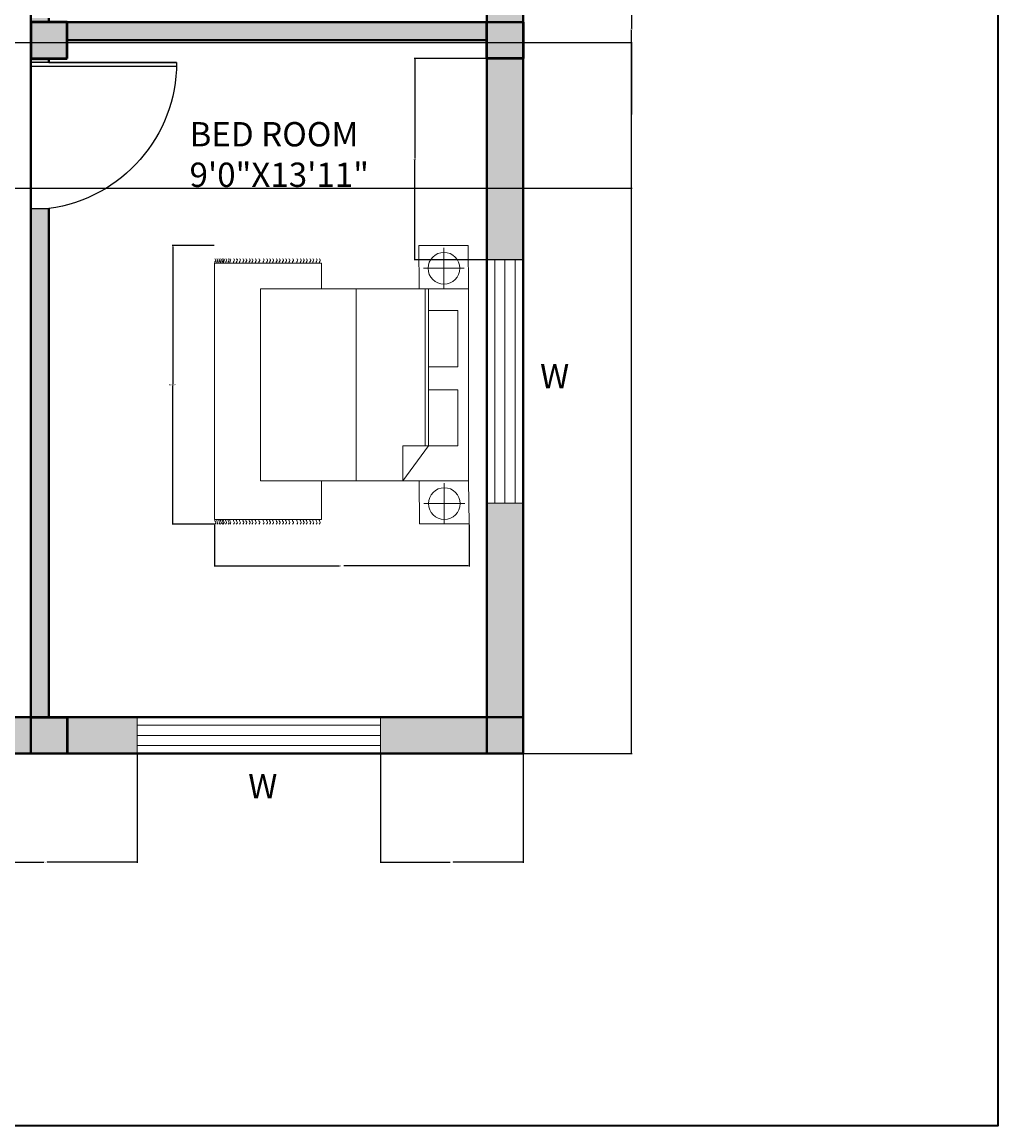
# Model space of a CAD drawing. Units: inches. Extents: x 25176543 to 25177243, y 80295576 to 80296086.
# Tile 6 of 11: x 25177002 to 25177243, y 80295576 to 80295848. Entities that reach past the tile are written whole.
import ezdxf

# ---------------------------------------------------------------- set-up
doc = ezdxf.new("R2010")
doc.units = ezdxf.units.IN
doc.header["$MEASUREMENT"] = 0
for name, color, linetype, lineweight in [('A-ANNO-DIMS', 2, 'Continuous', 18), ('A-ANNO-IDEN', 7, 'Continuous', 18), ('A-ANNO-TTLB', 7, 'Continuous', 35), ('A-AREA-IDEN', 7, 'Continuous', 18), ('A-COLS', 7, 'Continuous', 50), ('A-COLS-PATT', 251, 'Continuous', 13), ('A-DOOR', 3, 'Continuous', 25), ('A-GLAZ', 4, 'Continuous', 18), ('A-WALL', 7, 'Continuous', 40), ('A-WALL-PATT', 146, 'Continuous', 13), ('furniture', 31, 'Continuous', 13)]:
    doc.layers.add(name, color=color, linetype=linetype, lineweight=lineweight)
doc.styles.get("Standard").update_dxf_attribs({"font": 'arial.ttf'})
doc.dimstyles.get("Standard").update_dxf_attribs({"dimtxt": 0.18, "dimasz": 0.18, "dimexe": 0.18, "dimexo": 0.0625, "dimgap": 0.09, "dimtad": 0, "dimtih": 1, "dimtoh": 1, "dimdec": 4, "dimzin": 0, "dimdsep": 46, "dimtxsty": 'Standard', "dimcen": 0.09, "dimadec": 0, "dimazin": 0, "dimtfac": 1, "dimtdec": 4, "dimtofl": 0, "dimtmove": 0, "dimatfit": 3, "dimfxl": 1, "dimtolj": 1, "dimtzin": 0, "dimarcsym": 0})

# ---------------------------------------------------------------- blocks, each defined once
blk = doc.blocks.new('BED-DOUBLE-WITH-NIGHTSTANDS')
for p, q in [((5.6, 61.62), (5.6, 51.56)), ((63.65, 61.72), (63.65, 51.66)), ((10.63, 56.59), (0.57, 56.59)), ((68.68, 56.69), (58.62, 56.69)), ((49.39, 52.82), (10.63, 52.82)), ((49.44, 52), (10.63, 52)), ((49.39, 52.82), (58, 46.47)), ((49.44, 52.82), (49.44, 46.47)), ((49.44, 46.47), (58, 46.47)), ((58.05, 34.96), (10.63, 34.96)), ((4.35, 0), (4.35, 26.37)), ((4.35, 26.37), (10.65, 26.37)), ((58.05, 26.37), (67.59, 26.37)), ((67.59, 26.37), (67.59, 0)), ((67.59, 0), (4.35, 0))]:
    blk.add_line(p, q)
for points in [[(0, 50.39), (10.63, 50.5), (10.63, 62.68), (0, 62.58)], [(58.05, 62.68), (58.05, 11.37), (10.63, 11.37), (10.63, 62.68)], [(58.05, 50.5), (68.68, 50.6), (68.68, 62.78), (58.05, 62.68)], [(29.88, 59.98), (29.88, 52.82), (15.98, 52.82), (15.98, 59.98)], [(49.44, 59.98), (49.44, 52.82), (35.55, 52.82), (35.55, 59.98)]]:
    blk.add_lwpolyline(points, close=True)
for centre in [(5.6, 56.59), (63.65, 56.69)]:
    blk.add_circle(centre, 3.92)
for points, knots in [([(3.23, 25.84), (3.32, 25.96), (3.52, 26.2), (3.86, 25.96), (4.14, 25.78), (4.29, 25.89), (4.35, 25.94)], [0, 0, 0, 0, 0.400747, 0.791423, 1.067667, 1.29709, 1.29709, 1.29709, 1.29709]), ([(3.23, 25.06), (3.32, 25.18), (3.52, 25.42), (3.86, 25.18), (4.14, 25.01), (4.29, 25.11), (4.35, 25.16)], [0, 0, 0, 0, 0.400747, 0.791423, 1.067667, 1.29709, 1.29709, 1.29709, 1.29709]), ([(3.23, 24.24), (3.32, 24.36), (3.52, 24.6), (3.86, 24.36), (4.14, 24.19), (4.29, 24.3), (4.35, 24.34)], [0, 0, 0, 0, 0.400747, 0.791423, 1.067667, 1.29709, 1.29709, 1.29709, 1.29709]), ([(68.71, 25.84), (68.61, 25.96), (68.42, 26.2), (68.08, 25.96), (67.8, 25.78), (67.65, 25.89), (67.58, 25.94)], [0, 0, 0, 0, 0.400747, 0.791423, 1.067667, 1.29709, 1.29709, 1.29709, 1.29709]), ([(68.71, 25.06), (68.61, 25.18), (68.42, 25.42), (68.08, 25.18), (67.8, 25.01), (67.65, 25.11), (67.58, 25.16)], [0, 0, 0, 0, 0.400747, 0.791423, 1.067667, 1.29709, 1.29709, 1.29709, 1.29709]), ([(68.71, 24.24), (68.61, 24.36), (68.42, 24.6), (68.08, 24.36), (67.8, 24.19), (67.65, 24.3), (67.58, 24.34)], [0, 0, 0, 0, 0.400747, 0.791423, 1.067667, 1.29709, 1.29709, 1.29709, 1.29709]), ([(3.23, 23.51), (3.32, 23.63), (3.52, 23.87), (3.86, 23.63), (4.14, 23.46), (4.29, 23.57), (4.35, 23.62)], [0, 0, 0, 0, 0.400747, 0.791423, 1.067667, 1.29709, 1.29709, 1.29709, 1.29709]), ([(3.23, 22.63), (3.32, 22.75), (3.52, 22.99), (3.86, 22.75), (4.14, 22.58), (4.29, 22.69), (4.35, 22.73)], [0, 0, 0, 0, 0.400747, 0.791423, 1.067667, 1.29709, 1.29709, 1.29709, 1.29709]), ([(3.23, 21.88), (3.32, 22), (3.52, 22.24), (3.86, 22), (4.14, 21.83), (4.29, 21.93), (4.35, 21.98)], [0, 0, 0, 0, 0.400747, 0.791423, 1.067667, 1.29709, 1.29709, 1.29709, 1.29709]), ([(68.71, 23.51), (68.61, 23.63), (68.42, 23.87), (68.08, 23.63), (67.8, 23.46), (67.65, 23.57), (67.58, 23.62)], [0, 0, 0, 0, 0.400747, 0.791423, 1.067667, 1.29709, 1.29709, 1.29709, 1.29709]), ([(68.71, 22.63), (68.61, 22.75), (68.42, 22.99), (68.08, 22.75), (67.8, 22.58), (67.65, 22.69), (67.58, 22.73)], [0, 0, 0, 0, 0.400747, 0.791423, 1.067667, 1.29709, 1.29709, 1.29709, 1.29709]), ([(68.71, 21.88), (68.61, 22), (68.42, 22.24), (68.08, 22), (67.8, 21.83), (67.65, 21.93), (67.58, 21.98)], [0, 0, 0, 0, 0.400747, 0.791423, 1.067667, 1.29709, 1.29709, 1.29709, 1.29709]), ([(3.23, 21.15), (3.32, 21.27), (3.52, 21.51), (3.86, 21.27), (4.14, 21.1), (4.29, 21.21), (4.35, 21.25)], [0, 0, 0, 0, 0.400747, 0.791423, 1.067667, 1.29709, 1.29709, 1.29709, 1.29709]), ([(3.23, 20.27), (3.32, 20.39), (3.52, 20.63), (3.86, 20.39), (4.14, 20.22), (4.29, 20.32), (4.35, 20.37)], [0, 0, 0, 0, 0.400747, 0.791423, 1.067667, 1.29709, 1.29709, 1.29709, 1.29709]), ([(3.23, 19.23), (3.32, 19.35), (3.52, 19.59), (3.86, 19.35), (4.14, 19.18), (4.29, 19.29), (4.35, 19.33)], [0, 0, 0, 0, 0.400747, 0.791423, 1.067667, 1.29709, 1.29709, 1.29709, 1.29709]), ([(68.71, 21.15), (68.61, 21.27), (68.42, 21.51), (68.08, 21.27), (67.8, 21.1), (67.65, 21.21), (67.58, 21.25)], [0, 0, 0, 0, 0.400747, 0.791423, 1.067667, 1.29709, 1.29709, 1.29709, 1.29709]), ([(68.71, 20.27), (68.61, 20.39), (68.42, 20.63), (68.08, 20.39), (67.8, 20.22), (67.65, 20.32), (67.58, 20.37)], [0, 0, 0, 0, 0.400747, 0.791423, 1.067667, 1.29709, 1.29709, 1.29709, 1.29709]), ([(68.71, 19.23), (68.61, 19.35), (68.42, 19.59), (68.08, 19.35), (67.8, 19.18), (67.65, 19.29), (67.58, 19.33)], [0, 0, 0, 0, 0.400747, 0.791423, 1.067667, 1.29709, 1.29709, 1.29709, 1.29709]), ([(3.23, 18.35), (3.32, 18.47), (3.52, 18.71), (3.86, 18.47), (4.14, 18.3), (4.29, 18.4), (4.35, 18.45)], [0, 0, 0, 0, 0.400747, 0.791423, 1.067667, 1.29709, 1.29709, 1.29709, 1.29709]), ([(3.23, 17.53), (3.32, 17.65), (3.52, 17.89), (3.86, 17.65), (4.14, 17.48), (4.29, 17.59), (4.35, 17.64)], [0, 0, 0, 0, 0.400747, 0.791423, 1.067667, 1.29709, 1.29709, 1.29709, 1.29709]), ([(3.23, 16.76), (3.32, 16.88), (3.52, 17.12), (3.86, 16.88), (4.14, 16.7), (4.29, 16.81), (4.35, 16.86)], [0, 0, 0, 0, 0.400747, 0.791423, 1.067667, 1.29709, 1.29709, 1.29709, 1.29709]), ([(68.71, 18.35), (68.61, 18.47), (68.42, 18.71), (68.08, 18.47), (67.8, 18.3), (67.65, 18.4), (67.58, 18.45)], [0, 0, 0, 0, 0.400747, 0.791423, 1.067667, 1.29709, 1.29709, 1.29709, 1.29709]), ([(68.71, 17.53), (68.61, 17.65), (68.42, 17.89), (68.08, 17.65), (67.8, 17.48), (67.65, 17.59), (67.58, 17.64)], [0, 0, 0, 0, 0.400747, 0.791423, 1.067667, 1.29709, 1.29709, 1.29709, 1.29709]), ([(68.71, 16.76), (68.61, 16.88), (68.42, 17.12), (68.08, 16.88), (67.8, 16.7), (67.65, 16.81), (67.58, 16.86)], [0, 0, 0, 0, 0.400747, 0.791423, 1.067667, 1.29709, 1.29709, 1.29709, 1.29709]), ([(3.23, 15.94), (3.32, 16.06), (3.52, 16.3), (3.86, 16.06), (4.14, 15.89), (4.29, 16), (4.35, 16.04)], [0, 0, 0, 0, 0.400747, 0.791423, 1.067667, 1.29709, 1.29709, 1.29709, 1.29709]), ([(3.23, 15.21), (3.32, 15.33), (3.52, 15.57), (3.86, 15.33), (4.14, 15.16), (4.29, 15.27), (4.35, 15.32)], [0, 0, 0, 0, 0.400747, 0.791423, 1.067667, 1.29709, 1.29709, 1.29709, 1.29709]), ([(3.23, 14.33), (3.32, 14.45), (3.52, 14.69), (3.86, 14.45), (4.14, 14.28), (4.29, 14.38), (4.35, 14.43)], [0, 0, 0, 0, 0.400747, 0.791423, 1.067667, 1.29709, 1.29709, 1.29709, 1.29709]), ([(3.23, 13.58), (3.32, 13.7), (3.52, 13.94), (3.86, 13.7), (4.14, 13.53), (4.29, 13.63), (4.35, 13.68)], [0, 0, 0, 0, 0.400747, 0.791423, 1.067667, 1.29709, 1.29709, 1.29709, 1.29709]), ([(68.71, 15.94), (68.61, 16.06), (68.42, 16.3), (68.08, 16.06), (67.8, 15.89), (67.65, 16), (67.58, 16.04)], [0, 0, 0, 0, 0.400747, 0.791423, 1.067667, 1.29709, 1.29709, 1.29709, 1.29709]), ([(68.71, 15.21), (68.61, 15.33), (68.42, 15.57), (68.08, 15.33), (67.8, 15.16), (67.65, 15.27), (67.58, 15.32)], [0, 0, 0, 0, 0.400747, 0.791423, 1.067667, 1.29709, 1.29709, 1.29709, 1.29709]), ([(68.71, 14.33), (68.61, 14.45), (68.42, 14.69), (68.08, 14.45), (67.8, 14.28), (67.65, 14.38), (67.58, 14.43)], [0, 0, 0, 0, 0.400747, 0.791423, 1.067667, 1.29709, 1.29709, 1.29709, 1.29709]), ([(68.71, 13.58), (68.61, 13.7), (68.42, 13.94), (68.08, 13.7), (67.8, 13.53), (67.65, 13.63), (67.58, 13.68)], [0, 0, 0, 0, 0.400747, 0.791423, 1.067667, 1.29709, 1.29709, 1.29709, 1.29709]), ([(3.23, 12.85), (3.32, 12.97), (3.52, 13.21), (3.86, 12.97), (4.14, 12.8), (4.29, 12.9), (4.35, 12.95)], [0, 0, 0, 0, 0.400747, 0.791423, 1.067667, 1.29709, 1.29709, 1.29709, 1.29709]), ([(3.23, 11.97), (3.32, 12.09), (3.52, 12.33), (3.86, 12.09), (4.14, 11.92), (4.29, 12.02), (4.35, 12.07)], [0, 0, 0, 0, 0.400747, 0.791423, 1.067667, 1.29709, 1.29709, 1.29709, 1.29709]), ([(3.23, 10.93), (3.32, 11.05), (3.52, 11.29), (3.86, 11.05), (4.14, 10.88), (4.29, 10.99), (4.35, 11.03)], [0, 0, 0, 0, 0.400747, 0.791423, 1.067667, 1.29709, 1.29709, 1.29709, 1.29709]), ([(68.71, 12.85), (68.61, 12.97), (68.42, 13.21), (68.08, 12.97), (67.8, 12.8), (67.65, 12.9), (67.58, 12.95)], [0, 0, 0, 0, 0.400747, 0.791423, 1.067667, 1.29709, 1.29709, 1.29709, 1.29709]), ([(68.71, 11.97), (68.61, 12.09), (68.42, 12.33), (68.08, 12.09), (67.8, 11.92), (67.65, 12.02), (67.58, 12.07)], [0, 0, 0, 0, 0.400747, 0.791423, 1.067667, 1.29709, 1.29709, 1.29709, 1.29709]), ([(68.71, 10.93), (68.61, 11.05), (68.42, 11.29), (68.08, 11.05), (67.8, 10.88), (67.65, 10.99), (67.58, 11.03)], [0, 0, 0, 0, 0.400747, 0.791423, 1.067667, 1.29709, 1.29709, 1.29709, 1.29709]), ([(3.23, 10.05), (3.32, 10.17), (3.52, 10.41), (3.86, 10.17), (4.14, 10), (4.29, 10.1), (4.35, 10.15)], [0, 0, 0, 0, 0.400747, 0.791423, 1.067667, 1.29709, 1.29709, 1.29709, 1.29709]), ([(3.23, 9.23), (3.32, 9.35), (3.52, 9.59), (3.86, 9.35), (4.14, 9.18), (4.29, 9.29), (4.35, 9.34)], [0, 0, 0, 0, 0.400747, 0.791423, 1.067667, 1.29709, 1.29709, 1.29709, 1.29709]), ([(3.23, 8.54), (3.32, 8.66), (3.52, 8.9), (3.86, 8.66), (4.14, 8.49), (4.29, 8.6), (4.35, 8.65)], [0, 0, 0, 0, 0.400747, 0.791423, 1.067667, 1.29709, 1.29709, 1.29709, 1.29709]), ([(68.71, 10.05), (68.61, 10.17), (68.42, 10.41), (68.08, 10.17), (67.8, 10), (67.65, 10.1), (67.58, 10.15)], [0, 0, 0, 0, 0.400747, 0.791423, 1.067667, 1.29709, 1.29709, 1.29709, 1.29709]), ([(68.71, 9.23), (68.61, 9.35), (68.42, 9.59), (68.08, 9.35), (67.8, 9.18), (67.65, 9.29), (67.58, 9.34)], [0, 0, 0, 0, 0.400747, 0.791423, 1.067667, 1.29709, 1.29709, 1.29709, 1.29709]), ([(68.71, 8.54), (68.61, 8.66), (68.42, 8.9), (68.08, 8.66), (67.8, 8.49), (67.65, 8.6), (67.58, 8.65)], [0, 0, 0, 0, 0.400747, 0.791423, 1.067667, 1.29709, 1.29709, 1.29709, 1.29709]), ([(3.23, 7.73), (3.32, 7.85), (3.52, 8.09), (3.86, 7.85), (4.14, 7.68), (4.29, 7.78), (4.35, 7.83)], [0, 0, 0, 0, 0.400747, 0.791423, 1.067667, 1.29709, 1.29709, 1.29709, 1.29709]), ([(3.23, 7), (3.32, 7.12), (3.52, 7.36), (3.86, 7.12), (4.14, 6.95), (4.29, 7.05), (4.35, 7.1)], [0, 0, 0, 0, 0.400747, 0.791423, 1.067667, 1.29709, 1.29709, 1.29709, 1.29709]), ([(3.23, 6.12), (3.32, 6.24), (3.52, 6.48), (3.86, 6.24), (4.14, 6.07), (4.29, 6.17), (4.35, 6.22)], [0, 0, 0, 0, 0.400747, 0.791423, 1.067667, 1.29709, 1.29709, 1.29709, 1.29709]), ([(3.23, 5.36), (3.32, 5.49), (3.52, 5.73), (3.86, 5.49), (4.14, 5.31), (4.29, 5.42), (4.35, 5.47)], [0, 0, 0, 0, 0.400747, 0.791423, 1.067667, 1.29709, 1.29709, 1.29709, 1.29709]), ([(68.71, 7.73), (68.61, 7.85), (68.42, 8.09), (68.08, 7.85), (67.8, 7.68), (67.65, 7.78), (67.58, 7.83)], [0, 0, 0, 0, 0.400747, 0.791423, 1.067667, 1.29709, 1.29709, 1.29709, 1.29709]), ([(68.71, 7), (68.61, 7.12), (68.42, 7.36), (68.08, 7.12), (67.8, 6.95), (67.65, 7.05), (67.58, 7.1)], [0, 0, 0, 0, 0.400747, 0.791423, 1.067667, 1.29709, 1.29709, 1.29709, 1.29709]), ([(68.71, 6.12), (68.61, 6.24), (68.42, 6.48), (68.08, 6.24), (67.8, 6.07), (67.65, 6.17), (67.58, 6.22)], [0, 0, 0, 0, 0.400747, 0.791423, 1.067667, 1.29709, 1.29709, 1.29709, 1.29709]), ([(68.71, 5.36), (68.61, 5.49), (68.42, 5.73), (68.08, 5.49), (67.8, 5.31), (67.65, 5.42), (67.58, 5.47)], [0, 0, 0, 0, 0.400747, 0.791423, 1.067667, 1.29709, 1.29709, 1.29709, 1.29709]), ([(3.23, 4.64), (3.32, 4.76), (3.52, 5), (3.86, 4.76), (4.14, 4.59), (4.29, 4.69), (4.35, 4.74)], [0, 0, 0, 0, 0.400747, 0.791423, 1.067667, 1.29709, 1.29709, 1.29709, 1.29709]), ([(3.23, 3.75), (3.32, 3.88), (3.52, 4.12), (3.86, 3.88), (4.14, 3.7), (4.29, 3.81), (4.35, 3.86)], [0, 0, 0, 0, 0.400747, 0.791423, 1.067667, 1.29709, 1.29709, 1.29709, 1.29709]), ([(3.23, 3.33), (3.32, 3.45), (3.52, 3.7), (3.86, 3.44), (4.14, 3.27), (4.29, 3.38), (4.35, 3.43)], [0, 0, 0, 0, 0.407265, 0.802015, 1.07826, 1.307683, 1.307683, 1.307683, 1.307683]), ([(3.23, 2.76), (3.32, 2.88), (3.52, 3.12), (3.86, 2.88), (4.14, 2.71), (4.29, 2.81), (4.35, 2.86)], [0, 0, 0, 0, 0.400747, 0.791423, 1.067667, 1.29709, 1.29709, 1.29709, 1.29709]), ([(68.71, 4.64), (68.61, 4.76), (68.42, 5), (68.08, 4.76), (67.8, 4.59), (67.66, 4.69), (67.59, 4.73)], [0, 0, 0, 0, 0.400747, 0.791423, 1.067667, 1.283686, 1.283686, 1.283686, 1.283686]), ([(68.71, 3.75), (68.61, 3.88), (68.42, 4.11), (68.08, 3.88), (67.8, 3.7), (67.66, 3.81), (67.59, 3.85)], [0, 0, 0, 0, 0.400747, 0.791423, 1.067667, 1.283686, 1.283686, 1.283686, 1.283686]), ([(68.71, 3.33), (68.61, 3.45), (68.42, 3.69), (68.08, 3.45), (67.8, 3.27), (67.66, 3.38), (67.59, 3.42)], [0, 0, 0, 0, 0.402903, 0.794912, 1.071156, 1.287177, 1.287177, 1.287177, 1.287177]), ([(68.71, 2.73), (68.61, 2.85), (68.42, 3.09), (68.08, 2.85), (67.8, 2.68), (67.66, 2.78), (67.59, 2.82)], [0, 0, 0, 0, 0.400747, 0.791423, 1.067667, 1.283686, 1.283686, 1.283686, 1.283686]), ([(3.23, 2.18), (3.32, 2.31), (3.52, 2.55), (3.86, 2.31), (4.14, 2.13), (4.29, 2.24), (4.35, 2.29)], [0, 0, 0, 0, 0.400747, 0.791423, 1.067667, 1.29709, 1.29709, 1.29709, 1.29709]), ([(3.23, 1.88), (3.32, 2), (3.52, 2.24), (3.86, 2), (4.14, 1.82), (4.29, 1.93), (4.35, 1.98)], [0, 0, 0, 0, 0.400747, 0.791423, 1.067667, 1.29709, 1.29709, 1.29709, 1.29709]), ([(3.23, 1.46), (3.32, 1.58), (3.52, 1.82), (3.86, 1.58), (4.14, 1.41), (4.29, 1.51), (4.35, 1.56)], [0, 0, 0, 0, 0.400747, 0.791423, 1.067667, 1.29709, 1.29709, 1.29709, 1.29709]), ([(3.23, 1.06), (3.32, 1.18), (3.52, 1.42), (3.86, 1.18), (4.14, 1.01), (4.29, 1.11), (4.35, 1.16)], [0, 0, 0, 0, 0.400747, 0.791423, 1.067667, 1.29709, 1.29709, 1.29709, 1.29709]), ([(3.23, 0.57), (3.32, 0.7), (3.52, 0.94), (3.86, 0.7), (4.14, 0.52), (4.29, 0.63), (4.35, 0.68)], [0, 0, 0, 0, 0.400747, 0.791423, 1.067667, 1.29709, 1.29709, 1.29709, 1.29709]), ([(3.23, 0.07), (3.32, 0.19), (3.52, 0.43), (3.86, 0.19), (4.14, 0.02), (4.29, 0.13), (4.35, 0.18)], [0, 0, 0, 0, 0.400747, 0.791423, 1.067667, 1.29709, 1.29709, 1.29709, 1.29709]), ([(68.71, 1.43), (68.61, 1.55), (68.42, 1.79), (68.08, 1.55), (67.8, 1.38), (67.65, 1.48), (67.58, 1.53)], [0, 0, 0, 0, 0.400747, 0.791423, 1.067667, 1.29709, 1.29709, 1.29709, 1.29709]), ([(68.71, 1.03), (68.61, 1.15), (68.42, 1.39), (68.08, 1.15), (67.8, 0.98), (67.65, 1.09), (67.58, 1.13)], [0, 0, 0, 0, 0.400747, 0.791423, 1.067667, 1.29709, 1.29709, 1.29709, 1.29709]), ([(68.71, 0.55), (68.61, 0.67), (68.42, 0.91), (68.08, 0.67), (67.8, 0.49), (67.65, 0.6), (67.58, 0.65)], [0, 0, 0, 0, 0.400747, 0.791423, 1.067667, 1.29709, 1.29709, 1.29709, 1.29709]), ([(68.71, 0.07), (68.61, 0.19), (68.42, 0.43), (68.08, 0.19), (67.8, 0.02), (67.65, 0.13), (67.58, 0.18)], [0, 0, 0, 0, 0.400747, 0.791423, 1.067667, 1.29709, 1.29709, 1.29709, 1.29709]), ([(68.71, 2.16), (68.61, 2.28), (68.42, 2.52), (68.08, 2.28), (67.8, 2.11), (67.66, 2.21), (67.59, 2.25)], [0, 0, 0, 0, 0.400747, 0.791423, 1.067667, 1.283686, 1.283686, 1.283686, 1.283686]), ([(68.71, 1.85), (68.61, 1.97), (68.42, 2.21), (68.08, 1.97), (67.8, 1.8), (67.66, 1.9), (67.59, 1.94)], [0, 0, 0, 0, 0.400747, 0.791423, 1.067667, 1.283686, 1.283686, 1.283686, 1.283686])]:
    blk.add_open_spline(points, degree=3, knots=knots)
blk = doc.blocks.new('WIN-60IN')
for p, q in [((0, 9), (0, 0)), ((60, 9), (0, 9)), ((0, 9), (0, 4.5)), ((60, 0), (60, 9)), ((60, 7), (0, 7)), ((0, 4.5), (60, 4.5)), ((0, 2), (60, 2)), ((0, 0), (60, 0))]:
    blk.add_line(p, q)
blk = doc.blocks.new('DOOR-36IN-OFFSET')
for p, q in [((0, 1), (0, 37)), ((0, 37), (4.5, 37)), ((36, 2), (0, 2)), ((0, 0), (0, 1)), ((4.5, 1), (0, 1)), ((4.5, 1), (36, 1)), ((36, 1), (4.5, 1))]:
    blk.add_line(p, q)
blk.add_arc((-0.32, 1), 36.32, 0, 82.3719)
blk = doc.blocks.new('COLUMN-9IN-SQ')
for p, q in [((9, 9), (0, 9)), ((0, 9), (0, 0)), ((9, 0), (9, 9)), ((0, 0), (9, 0))]:
    blk.add_line(p, q)
blk = doc.blocks.new('*D28')
at = {"layer": 'A-ANNO-DIMS', "color": 0, "lineweight": -2, "transparency": 16777216}
for p, q in [((25177049.6, 80295793.15), (25177039.18, 80295793.15)), ((25177039.36, 80295792.97), (25177039.36, 80295758.98)), ((25177039.36, 80295724.62), (25177039.36, 80295758.61)), ((25177049.6, 80295724.44), (25177039.18, 80295724.44))]:
    blk.add_line(p, q, dxfattribs=at)
at = {"layer": 'A-ANNO-DIMS', "color": 0, "transparency": 16777216}
for points in [[(25177039.33, 80295792.97), (25177039.39, 80295792.97), (25177039.36, 80295793.15)], [(25177039.33, 80295724.62), (25177039.39, 80295724.62), (25177039.36, 80295724.44)]]:
    blk.add_solid(points, dxfattribs=at)
at = {"layer": 'Defpoints', "color": 0, "transparency": 16777216}
for p in [(25177049.66, 80295793.15), (25177039.36, 80295724.44), (25177049.66, 80295724.44)]:
    blk.add_point(p, dxfattribs=at)
at = {"layer": 'A-ANNO-DIMS', "color": 0, "transparency": 16777216, "insert": (25177039.36, 80295758.8), "char_height": 0.18, "attachment_point": 5}
blk.add_mtext('\\A1;BED SET 69 TYP.', dxfattribs=at)
blk = doc.blocks.new('*D29')
at = {"layer": 'A-ANNO-DIMS', "color": 0, "lineweight": -2, "transparency": 16777216}
for p, q in [((25177049.66, 80295724.38), (25177049.66, 80295713.95)), ((25177112.45, 80295724.38), (25177112.45, 80295713.95)), ((25177049.84, 80295714.13), (25177080.52, 80295714.13)), ((25177112.27, 80295714.13), (25177081.58, 80295714.13))]:
    blk.add_line(p, q, dxfattribs=at)
at = {"layer": 'A-ANNO-DIMS', "color": 0, "transparency": 16777216}
for points in [[(25177049.84, 80295714.16), (25177049.84, 80295714.1), (25177049.66, 80295714.13)], [(25177112.27, 80295714.16), (25177112.27, 80295714.1), (25177112.45, 80295714.13)]]:
    blk.add_solid(points, dxfattribs=at)
at = {"layer": 'Defpoints', "color": 0, "transparency": 16777216}
for p in [(25177049.66, 80295724.44), (25177112.45, 80295724.44), (25177112.45, 80295714.13)]:
    blk.add_point(p, dxfattribs=at)
at = {"layer": 'A-ANNO-DIMS', "color": 0, "transparency": 16777216, "insert": (25177081.05, 80295714.13), "char_height": 0.18, "attachment_point": 5}
blk.add_mtext('\\A1;63 TYP.', dxfattribs=at)
blk = doc.blocks.new('*D49')
at = {"layer": 'A-ANNO-DIMS', "color": 0, "lineweight": -2, "transparency": 16777216}
for p, q in [((25177125.86, 80296025.3), (25177152.73, 80296025.3)), ((25177152.55, 80296025.12), (25177152.55, 80295846.73)), ((25177152.55, 80295667.98), (25177152.55, 80295846.37)), ((25177125.86, 80295667.8), (25177152.73, 80295667.8))]:
    blk.add_line(p, q, dxfattribs=at)
at = {"layer": 'A-ANNO-DIMS', "color": 0, "transparency": 16777216}
for points in [[(25177152.52, 80296025.12), (25177152.58, 80296025.12), (25177152.55, 80296025.3)], [(25177152.52, 80295667.98), (25177152.58, 80295667.98), (25177152.55, 80295667.8)]]:
    blk.add_solid(points, dxfattribs=at)
at = {"layer": 'Defpoints', "color": 0, "transparency": 16777216}
for p in [(25177125.8, 80296025.3), (25177152.55, 80296025.3), (25177125.8, 80295667.8)]:
    blk.add_point(p, dxfattribs=at)
at = {"layer": 'A-ANNO-DIMS', "color": 0, "transparency": 16777216, "insert": (25177152.55, 80295846.55), "char_height": 0.18, "attachment_point": 5}
blk.add_mtext('\\A1;357.5', dxfattribs=at)
blk = doc.blocks.new('*D56')
at = {"layer": 'A-ANNO-DIMS', "color": 0, "lineweight": -2, "transparency": 16777216}
for p, q in [((25176985.3, 80295667.74), (25176985.3, 80295640.87)), ((25177030.59, 80295667.74), (25177030.59, 80295640.87)), ((25176985.48, 80295641.05), (25177007.55, 80295641.05)), ((25177030.41, 80295641.05), (25177008.34, 80295641.05))]:
    blk.add_line(p, q, dxfattribs=at)
at = {"layer": 'A-ANNO-DIMS', "color": 0, "transparency": 16777216}
for points in [[(25176985.48, 80295641.08), (25176985.48, 80295641.02), (25176985.3, 80295641.05)], [(25177030.41, 80295641.08), (25177030.41, 80295641.02), (25177030.59, 80295641.05)]]:
    blk.add_solid(points, dxfattribs=at)
at = {"layer": 'Defpoints', "color": 0, "transparency": 16777216}
for p in [(25176985.3, 80295667.8), (25177030.59, 80295667.8), (25177030.59, 80295641.05)]:
    blk.add_point(p, dxfattribs=at)
at = {"layer": 'A-ANNO-DIMS', "color": 0, "transparency": 16777216, "insert": (25177007.94, 80295641.05), "char_height": 0.18, "attachment_point": 5}
blk.add_mtext('\\A1;45.29', dxfattribs=at)
blk = doc.blocks.new('*D57')
at = {"layer": 'A-ANNO-DIMS', "color": 0, "lineweight": -2, "transparency": 16777216}
for p, q in [((25177090.59, 80295667.74), (25177090.59, 80295640.87)), ((25177125.8, 80295667.74), (25177125.8, 80295640.87)), ((25177090.77, 80295641.05), (25177107.82, 80295641.05)), ((25177125.62, 80295641.05), (25177108.57, 80295641.05))]:
    blk.add_line(p, q, dxfattribs=at)
at = {"layer": 'A-ANNO-DIMS', "color": 0, "transparency": 16777216}
for points in [[(25177090.77, 80295641.08), (25177090.77, 80295641.02), (25177090.59, 80295641.05)], [(25177125.62, 80295641.08), (25177125.62, 80295641.02), (25177125.8, 80295641.05)]]:
    blk.add_solid(points, dxfattribs=at)
at = {"layer": 'Defpoints', "color": 0, "transparency": 16777216}
for p in [(25177090.59, 80295667.8), (25177125.8, 80295667.8), (25177125.8, 80295641.05)]:
    blk.add_point(p, dxfattribs=at)
at = {"layer": 'A-ANNO-DIMS', "color": 0, "transparency": 16777216, "insert": (25177108.2, 80295641.05), "char_height": 0.18, "attachment_point": 5}
blk.add_mtext('\\A1;35.21', dxfattribs=at)
blk = doc.blocks.new('*D62')
at = {"layer": 'A-ANNO-DIMS', "color": 0, "lineweight": -2, "transparency": 16777216}
for p, q in [((25177125.74, 80295839.3), (25177098.87, 80295839.3)), ((25177099.05, 80295839.12), (25177099.05, 80295814.65)), ((25177099.05, 80295789.82), (25177099.05, 80295814.29)), ((25177125.74, 80295789.64), (25177098.87, 80295789.64))]:
    blk.add_line(p, q, dxfattribs=at)
at = {"layer": 'A-ANNO-DIMS', "color": 0, "transparency": 16777216}
for points in [[(25177099.02, 80295839.12), (25177099.08, 80295839.12), (25177099.05, 80295839.3)], [(25177099.02, 80295789.82), (25177099.08, 80295789.82), (25177099.05, 80295789.64)]]:
    blk.add_solid(points, dxfattribs=at)
at = {"layer": 'Defpoints', "color": 0, "transparency": 16777216}
for p in [(25177099.05, 80295839.3), (25177125.8, 80295839.3), (25177125.8, 80295789.64)]:
    blk.add_point(p, dxfattribs=at)
at = {"layer": 'A-ANNO-DIMS', "color": 0, "transparency": 16777216, "insert": (25177099.05, 80295814.47), "char_height": 0.18, "attachment_point": 5}
blk.add_mtext('\\A1;49.66', dxfattribs=at)
blk = doc.blocks.new('*D73')
at = {"layer": 'A-ANNO-DIMS', "color": 0, "lineweight": -2, "transparency": 16777216}
for p, q in [((25176791.86, 80295843.3), (25177152.73, 80295843.3)), ((25177152.55, 80295843.12), (25177152.55, 80295825.48)), ((25177152.55, 80295807.48), (25177152.55, 80295825.12)), ((25176791.86, 80295807.3), (25177152.73, 80295807.3))]:
    blk.add_line(p, q, dxfattribs=at)
at = {"layer": 'A-ANNO-DIMS', "color": 0, "transparency": 16777216}
for points in [[(25177152.52, 80295843.12), (25177152.58, 80295843.12), (25177152.55, 80295843.3)], [(25177152.52, 80295807.48), (25177152.58, 80295807.48), (25177152.55, 80295807.3)]]:
    blk.add_solid(points, dxfattribs=at)
at = {"layer": 'Defpoints', "color": 0, "transparency": 16777216}
for p in [(25176791.8, 80295843.3), (25177152.55, 80295843.3), (25176791.8, 80295807.3)]:
    blk.add_point(p, dxfattribs=at)
at = {"layer": 'A-ANNO-DIMS', "color": 0, "transparency": 16777216, "insert": (25177152.55, 80295825.3), "char_height": 0.18, "attachment_point": 5}
blk.add_mtext('\\A1;36', dxfattribs=at)

msp = doc.modelspace()

# ---------------------------------------------------------------- hatches: boundary and pattern name
at = {"layer": 'A-COLS-PATT'}
h = msp.add_hatch(color=256, dxfattribs=at)
h.dxf.hatch_style = 1
h.paths.add_polyline_path([(25176658.8016, 80296025.3022), (25176649.8016, 80296025.3022), (25176649.8016, 80296016.3022), (25176658.8016, 80296016.3022)])
h.paths.add_polyline_path([(25176819.3016, 80296025.3022), (25176810.3016, 80296025.3022), (25176810.3016, 80296016.3022), (25176819.3016, 80296016.3022)])
h.paths.add_polyline_path([(25176876.3016, 80296025.3022), (25176867.3016, 80296025.3022), (25176867.3016, 80296016.3022), (25176876.3016, 80296016.3022)])
h.paths.add_polyline_path([(25177013.3016, 80296025.3022), (25177004.3016, 80296025.3022), (25177004.3016, 80296016.3022), (25177013.3016, 80296016.3022)])
h.paths.add_polyline_path([(25176819.3016, 80295890.3022), (25176810.3016, 80295890.3022), (25176810.3016, 80295881.3022), (25176819.3016, 80295881.3022)])
h.paths.add_polyline_path([(25176658.8016, 80295890.3022), (25176649.8016, 80295890.3022), (25176649.8016, 80295881.3022), (25176658.8016, 80295881.3022)])
h.paths.add_polyline_path([(25177125.8016, 80296025.3022), (25177116.8016, 80296025.3022), (25177116.8016, 80296016.3022), (25177125.8016, 80296016.3022)])
h.paths.add_polyline_path([(25177125.8016, 80295848.3022), (25177116.8016, 80295848.3022), (25177116.8016, 80295839.3022), (25177125.8016, 80295839.3022)])
h.paths.add_polyline_path([(25177013.3016, 80295848.3022), (25177004.3016, 80295848.3022), (25177004.3016, 80295839.3022), (25177013.3016, 80295839.3022)])
h.paths.add_polyline_path([(25177125.8016, 80295676.8022), (25177116.8016, 80295676.8022), (25177116.8016, 80295667.8022), (25177125.8016, 80295667.8022)])
h.paths.add_polyline_path([(25177013.3016, 80295676.8022), (25177004.3016, 80295676.8022), (25177004.3016, 80295667.8022), (25177013.3016, 80295667.8022)])
h.paths.add_polyline_path([(25176842.3016, 80295676.8022), (25176833.3016, 80295676.8022), (25176833.3016, 80295667.8022), (25176842.3016, 80295667.8022)])
h.paths.add_polyline_path([(25176893.3016, 80295676.8022), (25176884.3016, 80295676.8022), (25176884.3016, 80295667.8022), (25176893.3016, 80295667.8022)])
h.paths.add_polyline_path([(25176842.3016, 80295807.3022), (25176833.3016, 80295807.3022), (25176833.3016, 80295798.3022), (25176842.3016, 80295798.3022)])
h.paths.add_polyline_path([(25176658.8016, 80295807.3022), (25176649.8016, 80295807.3022), (25176649.8016, 80295798.3022), (25176658.8016, 80295798.3022)])
h.paths.add_polyline_path([(25176658.8016, 80295676.8022), (25176649.8016, 80295676.8022), (25176649.8016, 80295667.8022), (25176658.8016, 80295667.8022)])
at = {"layer": 'A-WALL-PATT'}
h = msp.add_hatch(color=256, dxfattribs=at)
h.dxf.hatch_style = 1
h.paths.add_polyline_path([(25176695.189, 80296025.3022), (25176658.8016, 80296025.3022), (25176658.8016, 80296016.3022), (25176695.189, 80296016.3022)])
h.paths.add_polyline_path([(25176810.3016, 80296025.3022), (25176755.189, 80296025.3022), (25176755.189, 80296016.3022), (25176810.3016, 80296016.3022)])
h.paths.add_polyline_path([(25176819.3016, 80296016.3022), (25176814.8016, 80296016.3022), (25176814.8016, 80295965.3022), (25176819.3016, 80295965.3022)], flags=17)
h.paths.add_polyline_path([(25176828.0421, 80296025.3022), (25176819.3016, 80296025.3022), (25176819.3016, 80296016.3022), (25176828.0421, 80296016.3022)])
h.paths.add_polyline_path([(25176867.3016, 80296025.3022), (25176852.0421, 80296025.3022), (25176852.0421, 80296016.3022), (25176867.3016, 80296016.3022)])
h.paths.add_polyline_path([(25176885.1873, 80296025.3022), (25176876.3016, 80296025.3022), (25176876.3016, 80296016.3022), (25176885.1873, 80296016.3022)])
h.paths.add_polyline_path([(25176919.8016, 80296025.3022), (25176909.1873, 80296025.3022), (25176909.1873, 80296016.3022), (25176919.8016, 80296016.3022)])
h.paths.add_polyline_path([(25176924.3016, 80296016.3022), (25176919.8016, 80296016.3022), (25176919.8016, 80295890.3022), (25176904.8016, 80295890.3022), (25176904.8016, 80295885.8022), (25176967.3016, 80295885.8022), (25176967.3016, 80295890.3022), (25176924.3016, 80295890.3022)])
h.paths.add_polyline_path([(25176924.3016, 80296025.3022), (25176919.8016, 80296025.3022), (25176919.8016, 80296016.3022), (25176924.3016, 80296016.3022)])
h.paths.add_polyline_path([(25176938.7147, 80296025.3022), (25176924.3016, 80296025.3022), (25176924.3016, 80296016.3022), (25176938.7147, 80296016.3022)])
h.paths.add_polyline_path([(25176871.8016, 80296016.3022), (25176867.3016, 80296016.3022), (25176867.3016, 80295932.3022), (25176819.3016, 80295932.3022), (25176819.3016, 80295933.3022), (25176814.8016, 80295933.3022), (25176814.8016, 80295932.3022), (25176814.8016, 80295927.3022), (25176819.3016, 80295927.3022), (25176819.3016, 80295927.8022), (25176867.3016, 80295927.8022), (25176867.3016, 80295885.8022), (25176871.8016, 80295885.8022), (25176872.8016, 80295885.8022), (25176872.8016, 80295890.3022), (25176871.8016, 80295890.3022)])
h.paths.add_polyline_path([(25177004.3016, 80296025.3022), (25176986.7147, 80296025.3022), (25176986.7147, 80296016.3022), (25177004.3016, 80296016.3022)])
h.paths.add_polyline_path([(25177035.845, 80296025.3022), (25177013.3016, 80296025.3022), (25177013.3016, 80296016.3022), (25177035.845, 80296016.3022)])
h.paths.add_polyline_path([(25177008.8016, 80296016.3022), (25177004.3016, 80296016.3022), (25177004.3016, 80295890.3022), (25177003.3016, 80295890.3022), (25177003.3016, 80295885.8022), (25177004.3016, 80295885.8022), (25177004.3016, 80295885.3022), (25177008.8016, 80295885.3022)])
h.paths.add_polyline_path([(25177116.8016, 80296025.3022), (25177095.845, 80296025.3022), (25177095.845, 80296016.3022), (25177116.8016, 80296016.3022)])
h.paths.add_polyline_path([(25177125.8016, 80296016.3022), (25177116.8016, 80296016.3022), (25177116.8016, 80295971.1334), (25177121.3016, 80295971.1334), (25177125.8016, 80295971.1334)])
h.paths.add_polyline_path([(25177116.8016, 80295848.3022), (25177013.3016, 80295848.3022), (25177013.3016, 80295843.8022), (25177116.8016, 80295843.8022)])
h.paths.add_polyline_path([(25177125.8016, 80295911.1334), (25177116.8016, 80295911.1334), (25177116.8016, 80295848.3022), (25177125.8016, 80295848.3022)])
h.paths.add_polyline_path([(25177008.8016, 80295802.3022), (25177004.3016, 80295802.3022), (25177004.3016, 80295676.8022), (25177008.8016, 80295676.8022)])
h.paths.add_polyline_path([(25176658.8016, 80295705.5694), (25176649.8016, 80295705.5694), (25176649.8016, 80295676.8022), (25176658.8016, 80295676.8022)])
h.paths.add_polyline_path([(25176658.8016, 80295798.3022), (25176649.8016, 80295798.3022), (25176649.8016, 80295765.5694), (25176654.3016, 80295765.5694), (25176658.8016, 80295765.5694)])
h.paths.add_polyline_path([(25176833.3016, 80295807.3022), (25176658.8016, 80295807.3022), (25176658.8016, 80295802.8022), (25176833.3016, 80295802.8022)])
h.paths.add_polyline_path([(25176842.3016, 80295761.3022), (25176837.8016, 80295761.3022), (25176837.8016, 80295676.8022), (25176842.3016, 80295676.8022)])
h.paths.add_polyline_path([(25176649.8016, 80295807.3022), (25176629.8016, 80295807.3022), (25176629.8016, 80295885.8022), (25176649.8016, 80295885.8022), (25176649.8016, 80295890.3022), (25176625.3016, 80295890.3022), (25176625.3016, 80295802.8022), (25176649.8016, 80295802.8022)])
h.paths.add_polyline_path([(25176810.3016, 80295890.3022), (25176658.8016, 80295890.3022), (25176658.8016, 80295885.8022), (25176810.3016, 80295885.8022)])
h.paths.add_polyline_path([(25176658.8016, 80295922.9263), (25176649.8016, 80295922.9263), (25176649.8016, 80295890.3022), (25176658.8016, 80295890.3022)])
h.paths.add_polyline_path([(25176658.8016, 80296016.3022), (25176649.8016, 80296016.3022), (25176649.8016, 80295982.9263), (25176654.3016, 80295982.9263), (25176658.8016, 80295982.9263)])
h = msp.add_hatch(color=256, dxfattribs=at)
h.dxf.hatch_style = 1
h.paths.add_polyline_path([(25177008.8016, 80295839.3022), (25177004.3016, 80295839.3022), (25177004.3016, 80295838.3022), (25177008.8016, 80295838.3022)])
h.paths.add_polyline_path([(25177008.8016, 80295849.3022), (25177004.3016, 80295849.3022), (25177004.3016, 80295848.3022), (25177008.8016, 80295848.3022)])
h = msp.add_hatch(color=256, dxfattribs=at)
h.dxf.hatch_style = 1
h.paths.add_polyline_path([(25176705.5738, 80295676.8022), (25176658.8016, 80295676.8022), (25176658.8016, 80295667.8022), (25176705.5738, 80295667.8022)])
h.paths.add_polyline_path([(25176833.3016, 80295676.8022), (25176765.5738, 80295676.8022), (25176765.5738, 80295667.8022), (25176833.3016, 80295667.8022)])
h.paths.add_polyline_path([(25176925.2997, 80295676.8022), (25176893.3016, 80295676.8022), (25176893.3016, 80295667.8022), (25176925.2997, 80295667.8022)])
h.paths.add_polyline_path([(25177004.3016, 80295676.8022), (25176985.2997, 80295676.8022), (25176985.2997, 80295667.8022), (25177004.3016, 80295667.8022)])
h.paths.add_polyline_path([(25177030.5901, 80295676.8022), (25177013.3016, 80295676.8022), (25177013.3016, 80295667.8022), (25177030.5901, 80295667.8022)])
h.paths.add_polyline_path([(25177116.8016, 80295676.8022), (25177090.5901, 80295676.8022), (25177090.5901, 80295667.8022), (25177116.8016, 80295667.8022)])
h.paths.add_polyline_path([(25177125.8016, 80295729.6384), (25177116.8016, 80295729.6384), (25177116.8016, 80295676.8022), (25177125.8016, 80295676.8022)])
h.paths.add_polyline_path([(25177125.8016, 80295839.3022), (25177116.8016, 80295839.3022), (25177116.8016, 80295789.6384), (25177121.3016, 80295789.6384), (25177125.8016, 80295789.6384)])

# ---------------------------------------------------------------- linework, layer by layer
at = {"layer": 'A-ANNO-TTLB'}
msp.add_lwpolyline([(25176542.8973, 80296086.2335), (25177242.9194, 80296086.2335), (25177242.9194, 80295575.9501), (25176542.8973, 80295575.9501)], close=True, dxfattribs=at)
at = {"layer": 'A-COLS'}
for p, q in [((25177116.8016, 80295839.3022), (25177116.8016, 80295848.3022)), ((25177125.8016, 80295848.3022), (25177125.8016, 80295839.3022)), ((25177125.8016, 80295839.3022), (25177116.8016, 80295839.3022)), ((25177004.3016, 80295676.8022), (25177013.3016, 80295676.8022)), ((25177013.3016, 80295676.8022), (25177013.3016, 80295667.8022))]:
    msp.add_line(p, q, dxfattribs=at)
at = {"layer": 'A-GLAZ'}
msp.add_line((25177116.8016, 80295729.6384), (25177116.8016, 80295729.6384), dxfattribs=at)
at = {"layer": 'A-WALL'}
for p, q in [((25177116.8016, 80296025.3022), (25177116.8016, 80295667.8022)), ((25177125.8016, 80296025.3022), (25177125.8016, 80295667.8022)), ((25177004.3016, 80295885.8022), (25177004.3016, 80295667.8022)), ((25177008.8016, 80295849.3022), (25177008.8016, 80295848.3022)), ((25177004.3016, 80295848.3022), (25177125.8016, 80295848.3022)), ((25177013.3016, 80295843.8022), (25177116.8016, 80295843.8022)), ((25177008.8016, 80295839.3022), (25177008.8016, 80295838.3022)), ((25177008.8016, 80295802.3022), (25177008.8016, 80295676.8022)), ((25177004.3016, 80295676.8022), (25177004.3016, 80295677.8022)), ((25176884.3016, 80295676.8022), (25177125.8016, 80295676.8022)), ((25176649.8016, 80295667.8022), (25177125.8016, 80295667.8022))]:
    msp.add_line(p, q, dxfattribs=at)

# ---------------------------------------------------------------- block references
at = {"layer": 'A-COLS', "rotation": 90.0000001422956}
msp.add_blockref('COLUMN-9IN-SQ', (25177013.3018, 80295839.3026), dxfattribs=at)
at = {"layer": 'A-DOOR', "extrusion": (0, 0, -1), "zscale": -1, "rotation": 180}
msp.add_blockref('DOOR-36IN-OFFSET', (-25177004.302, 80295839.3024), dxfattribs=at)
at = {"layer": 'A-GLAZ', "extrusion": (0, 0, -1), "zscale": -1, "rotation": 270.000000047842}
msp.add_blockref('WIN-60IN', (-25177125.8018, 80295789.6385), dxfattribs=at)
at = {"layer": 'A-GLAZ'}
msp.add_blockref('WIN-60IN', (25177030.5901, 80295667.802), dxfattribs=at)
at = {"layer": 'furniture', "rotation": 269.9999998239466}
msp.add_blockref('BED-DOUBLE-WITH-NIGHTSTANDS', (25177049.6616, 80295793.1502), dxfattribs=at)

# ---------------------------------------------------------------- texts
at = {"layer": 'A-ANNO-IDEN', "char_height": 6, "attachment_point": 1}
for insert in [(25177129.9709, 80295763.9468), (25177057.975, 80295662.7705)]:
    msp.add_mtext_dynamic_manual_height_columns('W', width=24.139595, gutter_width=1, heights=[0], dxfattribs=dict(at, insert=insert))
at = {"layer": 'A-AREA-IDEN', "insert": (25177043.4953, 80295823.632), "char_height": 6, "attachment_point": 1}
msp.add_mtext_dynamic_manual_height_columns('BED ROOM\\P9\'0"X13\'11"', width=51.655639, gutter_width=1, heights=[0], dxfattribs=at)

# ---------------------------------------------------------------- dimensions: what is measured, and where the dimension line sits
at = {"layer": 'A-ANNO-DIMS'}
for base, p1, p2, override, picture, middle in [((25177152.5516, 80296025.3022), (25177125.8016, 80295667.8022), (25177125.8016, 80296025.3022), {"dimdec": 1, "dimlfac": 1, "dimrnd": 0, "dimzin": 0, "dimdsep": 46, "dimlunit": 2}, '*D49', (25177152.5516, 80295846.5522)), ((25177152.5516, 80295843.3022), (25176791.8016, 80295807.3022), (25176791.8016, 80295843.3022), {"dimdec": 0, "dimlfac": 1, "dimrnd": 0, "dimzin": 0, "dimdsep": 46, "dimlunit": 2}, '*D73', (25177152.5516, 80295825.3022)), ((25177099.0516, 80295839.3022), (25177125.8016, 80295789.6384), (25177125.8016, 80295839.3022), {"dimdec": 2, "dimlfac": 1, "dimrnd": 0, "dimzin": 0, "dimdsep": 46, "dimlunit": 2}, '*D62', (25177099.0516, 80295814.4703))]:
    dim = msp.add_linear_dim(base=base, p1=p1, p2=p2, angle=90, dimstyle='Standard', override=override, dxfattribs=at)
    dim.commit()
    dim.dimension.update_dxf_attribs({"geometry": picture, "text_midpoint": middle})
for base, p1, p2, angle, text, picture, middle in [((25177039.3553, 80295724.4402), (25177049.6618, 80295793.1501), (25177049.6618, 80295724.4402), 270, 'BED SET <> TYP.', '*D28', (25177039.3553, 80295758.7951)), ((25177112.4453, 80295714.1337), (25177049.6618, 80295724.4402), (25177112.4453, 80295724.4402), 360, '<> TYP.', '*D29', (25177081.0536, 80295714.1337))]:
    dim = msp.add_linear_dim(base=base, p1=p1, p2=p2, angle=angle, text=text, dimstyle='Standard', override={"dimdec": 0, "dimlfac": 1, "dimrnd": 0, "dimzin": 0, "dimdsep": 46, "dimlunit": 2}, dxfattribs=at)
    dim.commit()
    dim.dimension.update_dxf_attribs({"geometry": picture, "text_midpoint": middle})
for base, p1, p2, picture, middle in [((25177030.5901, 80295641.0522), (25176985.2997, 80295667.8022), (25177030.5901, 80295667.8022), '*D56', (25177007.9449, 80295641.0522)), ((25177125.8016, 80295641.0522), (25177090.5901, 80295667.8022), (25177125.8016, 80295667.8022), '*D57', (25177108.1958, 80295641.0522))]:
    dim = msp.add_linear_dim(base=base, p1=p1, p2=p2, dimstyle='Standard', override={"dimdec": 2, "dimlfac": 1, "dimrnd": 0, "dimzin": 0, "dimdsep": 46, "dimlunit": 2}, dxfattribs=at)
    dim.commit()
    dim.dimension.update_dxf_attribs({"geometry": picture, "text_midpoint": middle})

doc.saveas('drawing.dxf')
